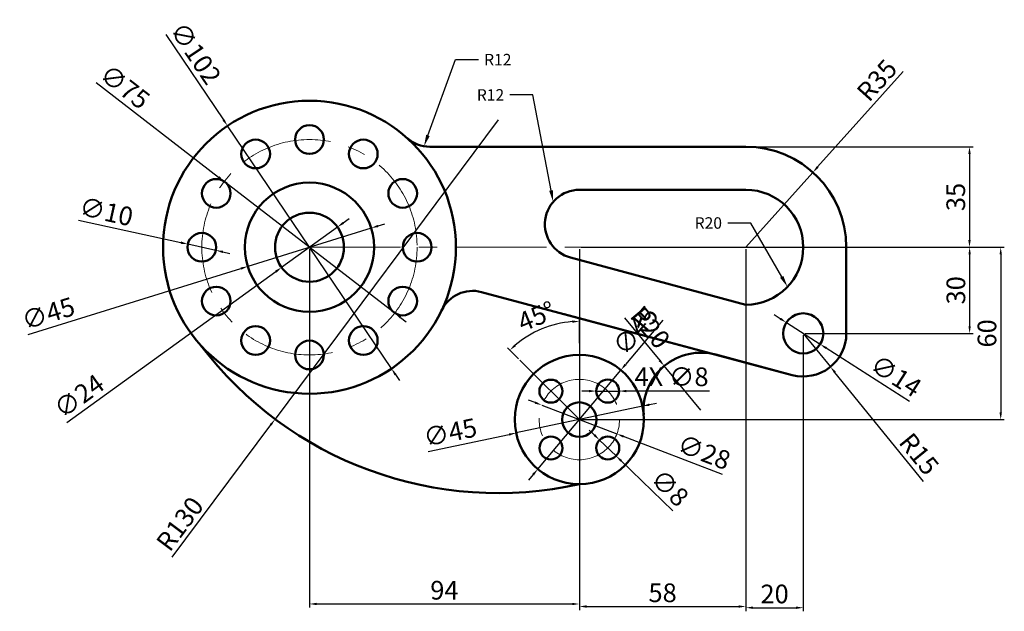
# Model space of a CAD drawing. Units: millimetres. Extents: x 3100 to 3443, y 1438 to 1644.
import ezdxf
from ezdxf import colors
from ezdxf.entities.mleader import LeaderData, LeaderLine
from ezdxf.math import Vec2, Vec3

# ---------------------------------------------------------------- set-up
doc = ezdxf.new("R2010")
doc.units = ezdxf.units.MM
doc.linetypes.add('CENTER', pattern=[50.8, 31.75, -6.35, 6.35, -6.35])
for name, color, linetype, lineweight in [('M-CNTR', 240, 'CENTER', 18), ('M-DIMS', 2, 'Continuous', 25), ('M-OUTL', 7, 'Continuous', 50)]:
    doc.layers.add(name, color=color, linetype=linetype, lineweight=lineweight)
doc.styles.get("Standard").update_dxf_attribs({"font": 'arial.ttf'})
doc.dimstyles.new('ISO-25', dxfattribs={"dimtxt": 6.5, "dimasz": 2.5, "dimexe": 1.25, "dimexo": 0.625, "dimtad": 1, "dimtxsty": 'Standard', "dimcen": 2.5, "dimadec": 0, "dimazin": 0, "dimtfac": 1, "dimtmove": 0, "dimatfit": 3, "dimfxl": 1, "dimarcsym": 0})

# ---------------------------------------------------------------- blocks, each defined once
blk = doc.blocks.new('*D1')
at = {"layer": 'Defpoints', "color": 0, "transparency": 16777216}
for p in [(3372.48, 1564.51), (3372.48, 1534.51), (3430.43, 1534.51)]:
    blk.add_point(p, dxfattribs=at)
at = {"layer": 'M-DIMS', "color": 0, "lineweight": -2, "transparency": 16777216}
for p, q in [((3373.1, 1564.51), (3431.68, 1564.51)), ((3430.43, 1562.01), (3430.43, 1537.01)), ((3373.1, 1534.51), (3431.68, 1534.51))]:
    blk.add_line(p, q, dxfattribs=at)
at = {"layer": 'M-DIMS', "color": 0, "transparency": 16777216}
for points in [[(3430.01, 1562.01), (3430.84, 1562.01), (3430.43, 1564.51)], [(3430.01, 1537.01), (3430.84, 1537.01), (3430.43, 1534.51)]]:
    blk.add_solid(points, dxfattribs=at)
at = {"layer": 'M-DIMS', "color": 0, "transparency": 16777216, "insert": (3426.48, 1549.51), "char_height": 6.5, "attachment_point": 5, "rotation": 90}
blk.add_mtext('30', dxfattribs=at)
blk = doc.blocks.new('*D2')
at = {"layer": 'Defpoints', "color": 0, "transparency": 16777216}
for p in [(3352.48, 1564.51), (3372.48, 1534.51), (3372.48, 1438.99)]:
    blk.add_point(p, dxfattribs=at)
at = {"layer": 'M-DIMS', "color": 0, "lineweight": -2, "transparency": 16777216}
for p, q in [((3352.48, 1563.88), (3352.48, 1437.74)), ((3372.48, 1533.88), (3372.48, 1437.74)), ((3354.98, 1438.99), (3369.98, 1438.99))]:
    blk.add_line(p, q, dxfattribs=at)
at = {"layer": 'M-DIMS', "color": 0, "transparency": 16777216}
for points in [[(3354.98, 1439.41), (3354.98, 1438.58), (3352.48, 1438.99)], [(3369.98, 1439.41), (3369.98, 1438.58), (3372.48, 1438.99)]]:
    blk.add_solid(points, dxfattribs=at)
at = {"layer": 'M-DIMS', "color": 0, "transparency": 16777216, "insert": (3362.48, 1442.94), "char_height": 6.5, "attachment_point": 5}
blk.add_mtext('20', dxfattribs=at)
blk = doc.blocks.new('*D3')
at = {"layer": 'Defpoints', "color": 0, "transparency": 16777216}
for p in [(3331.88, 1599.51), (3352.09, 1564.51), (3430.38, 1564.51)]:
    blk.add_point(p, dxfattribs=at)
at = {"layer": 'M-DIMS', "color": 0, "lineweight": -2, "transparency": 16777216}
for p, q in [((3332.51, 1599.51), (3431.63, 1599.51)), ((3430.38, 1597.01), (3430.38, 1567.01)), ((3352.72, 1564.51), (3431.63, 1564.51))]:
    blk.add_line(p, q, dxfattribs=at)
at = {"layer": 'M-DIMS', "color": 0, "transparency": 16777216}
for points in [[(3429.97, 1597.01), (3430.8, 1597.01), (3430.38, 1599.51)], [(3429.97, 1567.01), (3430.8, 1567.01), (3430.38, 1564.51)]]:
    blk.add_solid(points, dxfattribs=at)
at = {"layer": 'M-DIMS', "color": 0, "transparency": 16777216, "insert": (3426.44, 1582.01), "char_height": 6.5, "attachment_point": 5, "rotation": 90}
blk.add_mtext('35', dxfattribs=at)
blk = doc.blocks.new('*D4')
at = {"layer": 'Defpoints', "color": 0, "transparency": 16777216}
for p in [(3171.92, 1606.77), (3229.03, 1522.25)]:
    blk.add_point(p, dxfattribs=at)
at = {"layer": 'M-DIMS', "color": 0, "lineweight": -2, "transparency": 16777216}
for p, q in [((3150.4, 1638.62), (3170.53, 1608.84)), ((3229.03, 1522.25), (3171.92, 1606.77)), ((3230.43, 1520.18), (3231.83, 1518.11))]:
    blk.add_line(p, q, dxfattribs=at)
at = {"layer": 'M-DIMS', "color": 0, "transparency": 16777216}
for points in [[(3170.87, 1609.07), (3170.18, 1608.6), (3171.92, 1606.77)], [(3230.77, 1520.41), (3230.08, 1519.94), (3229.03, 1522.25)]]:
    blk.add_solid(points, dxfattribs=at)
at = {"layer": 'M-DIMS', "color": 0, "transparency": 16777216, "insert": (3160.15, 1631.56), "char_height": 6.5, "attachment_point": 5, "rotation": 304.0444}
blk.add_mtext('∅102', dxfattribs=at)
blk = doc.blocks.new('*D5')
at = {"layer": 'Defpoints', "color": 0, "transparency": 16777216}
for p in [(3170.78, 1587.41), (3230.17, 1541.61)]:
    blk.add_point(p, dxfattribs=at)
at = {"layer": 'M-DIMS', "color": 0, "lineweight": -2, "transparency": 16777216}
for p, q in [((3126.15, 1621.82), (3168.8, 1588.93)), ((3230.17, 1541.61), (3170.78, 1587.41)), ((3232.15, 1540.08), (3234.13, 1538.55))]:
    blk.add_line(p, q, dxfattribs=at)
at = {"layer": 'M-DIMS', "color": 0, "transparency": 16777216}
for points in [[(3169.06, 1589.26), (3168.55, 1588.6), (3170.78, 1587.41)], [(3232.41, 1540.41), (3231.9, 1539.75), (3230.17, 1541.61)]]:
    blk.add_solid(points, dxfattribs=at)
at = {"layer": 'M-DIMS', "color": 0, "transparency": 16777216, "insert": (3135.67, 1619.69), "char_height": 6.5, "attachment_point": 5, "rotation": 322.3623}
blk.add_mtext('∅75', dxfattribs=at)
blk = doc.blocks.new('*D6')
at = {"layer": 'Defpoints', "color": 0, "transparency": 16777216}
for p in [(3158.09, 1565.58), (3167.86, 1563.43)]:
    blk.add_point(p, dxfattribs=at)
at = {"layer": 'M-DIMS', "color": 0, "lineweight": -2, "transparency": 16777216}
for p, q in [((3120.04, 1573.96), (3155.65, 1566.12)), ((3167.86, 1563.43), (3158.09, 1565.58)), ((3170.3, 1562.9), (3172.74, 1562.36))]:
    blk.add_line(p, q, dxfattribs=at)
at = {"layer": 'M-DIMS', "color": 0, "transparency": 16777216}
for points in [[(3155.74, 1566.53), (3155.56, 1565.71), (3158.09, 1565.58)], [(3170.39, 1563.3), (3170.21, 1562.49), (3167.86, 1563.43)]]:
    blk.add_solid(points, dxfattribs=at)
at = {"layer": 'M-DIMS', "color": 0, "transparency": 16777216, "insert": (3129.53, 1576.1), "char_height": 6.5, "attachment_point": 5, "rotation": 347.5819}
blk.add_mtext('∅10', dxfattribs=at)
blk = doc.blocks.new('*D7')
at = {"layer": 'Defpoints', "color": 0, "transparency": 16777216}
for p in [(3221.96, 1571.18), (3178.99, 1557.84)]:
    blk.add_point(p, dxfattribs=at)
at = {"layer": 'M-DIMS', "color": 0, "lineweight": -2, "transparency": 16777216}
for p, q in [((3221.96, 1571.18), (3178.99, 1557.84)), ((3224.35, 1571.92), (3226.74, 1572.66)), ((3102.51, 1534.1), (3176.6, 1557.1))]:
    blk.add_line(p, q, dxfattribs=at)
at = {"layer": 'M-DIMS', "color": 0, "transparency": 16777216}
for points in [[(3224.23, 1572.32), (3224.48, 1571.52), (3221.96, 1571.18)], [(3176.48, 1557.49), (3176.72, 1556.7), (3178.99, 1557.84)]]:
    blk.add_solid(points, dxfattribs=at)
at = {"layer": 'M-DIMS', "color": 0, "transparency": 16777216, "insert": (3109.73, 1540.66), "char_height": 6.5, "attachment_point": 5, "rotation": 17.2442}
blk.add_mtext('∅45', dxfattribs=at)
blk = doc.blocks.new('*D8')
at = {"layer": 'Defpoints', "color": 0, "transparency": 16777216}
for p in [(3210.21, 1571.53), (3190.75, 1557.48)]:
    blk.add_point(p, dxfattribs=at)
at = {"layer": 'M-DIMS', "color": 0, "lineweight": -2, "transparency": 16777216}
for p, q in [((3212.23, 1572.99), (3214.26, 1574.46)), ((3210.21, 1571.53), (3190.75, 1557.48)), ((3115.96, 1503.5), (3188.72, 1556.02))]:
    blk.add_line(p, q, dxfattribs=at)
at = {"layer": 'M-DIMS', "color": 0, "transparency": 16777216}
for points in [[(3211.99, 1573.33), (3212.48, 1572.66), (3210.21, 1571.53)], [(3188.48, 1556.36), (3188.96, 1555.68), (3190.75, 1557.48)]]:
    blk.add_solid(points, dxfattribs=at)
at = {"layer": 'M-DIMS', "color": 0, "transparency": 16777216, "insert": (3120.68, 1512), "char_height": 6.5, "attachment_point": 5, "rotation": 35.823}
blk.add_mtext('∅24', dxfattribs=at)
blk = doc.blocks.new('*D9')
at = {"layer": 'Defpoints', "color": 0, "transparency": 16777216}
for p in [(3266.19, 1608.89), (3188.49, 1504.67)]:
    blk.add_point(p, dxfattribs=at)
at = {"layer": 'M-DIMS', "color": 0, "lineweight": -2, "transparency": 16777216}
for p, q in [((3266.19, 1608.89), (3188.49, 1504.67)), ((3152.65, 1456.59), (3186.99, 1502.66))]:
    blk.add_line(p, q, dxfattribs=at)
at = {"layer": 'M-DIMS', "color": 0, "transparency": 16777216}
blk.add_solid([(3186.66, 1502.91), (3187.33, 1502.41), (3188.49, 1504.67)], dxfattribs=at)
at = {"layer": 'M-DIMS', "color": 0, "transparency": 16777216, "insert": (3156, 1467.69), "char_height": 6.5, "attachment_point": 5, "rotation": 53.2956}
blk.add_mtext('R130', dxfattribs=at)
blk = doc.blocks.new('*D10')
at = {"layer": 'Defpoints', "color": 0, "transparency": 16777216}
for p in [(3375.82, 1590.58), (3352.48, 1564.51)]:
    blk.add_point(p, dxfattribs=at)
at = {"layer": 'M-DIMS', "color": 0, "lineweight": -2, "transparency": 16777216}
for p, q in [((3407.31, 1625.75), (3377.49, 1592.45)), ((3352.48, 1564.51), (3375.82, 1590.58))]:
    blk.add_line(p, q, dxfattribs=at)
at = {"layer": 'M-DIMS', "color": 0, "transparency": 16777216}
blk.add_solid([(3377.18, 1592.72), (3377.8, 1592.17), (3375.82, 1590.58)], dxfattribs=at)
at = {"layer": 'M-DIMS', "color": 0, "transparency": 16777216, "insert": (3398.76, 1622.11), "char_height": 6.5, "attachment_point": 5, "rotation": 48.1595}
blk.add_mtext('R35', dxfattribs=at)
blk = doc.blocks.new('*D11')
at = {"layer": 'Defpoints', "color": 0, "transparency": 16777216}
for p in [(3285.62, 1537.52), (3294.48, 1530.53), (3273.7, 1525.24), (3294.48, 1504.51), (3294.48, 1504.51)]:
    blk.add_point(p, dxfattribs=at)
at = {"layer": 'M-DIMS', "color": 0, "lineweight": -2, "transparency": 16777216}
for p, q in [((3294.48, 1531.16), (3294.48, 1539.94)), ((3273.26, 1525.68), (3269.4, 1529.53))]:
    blk.add_line(p, q, dxfattribs=at)
blk.add_arc((3294.48, 1504.51), 34.18, 94.192, 130.8751, dxfattribs=at)
at = {"layer": 'M-DIMS', "color": 0, "transparency": 16777216}
for points in [[(3291.96, 1539.01), (3291.99, 1538.18), (3294.48, 1538.69)], [(3272.39, 1530.05), (3271.83, 1530.66), (3270.28, 1528.65)]]:
    blk.add_solid(points, dxfattribs=at)
at = {"layer": 'M-DIMS', "color": 0, "transparency": 16777216, "insert": (3279.87, 1539.71), "char_height": 6.5, "attachment_point": 5, "rotation": 22.5336}
blk.add_mtext('45°', dxfattribs=at)
blk = doc.blocks.new('*D12')
at = {"layer": 'Defpoints', "color": 0, "transparency": 16777216}
for p in [(3200.48, 1564.51), (3294.48, 1564.51), (3294.48, 1440.29)]:
    blk.add_point(p, dxfattribs=at)
at = {"layer": 'M-DIMS', "color": 0, "lineweight": -2, "transparency": 16777216}
for p, q in [((3200.48, 1563.88), (3200.48, 1439.04)), ((3294.48, 1563.88), (3294.48, 1439.04)), ((3202.98, 1440.29), (3291.98, 1440.29))]:
    blk.add_line(p, q, dxfattribs=at)
at = {"layer": 'M-DIMS', "color": 0, "transparency": 16777216}
for points in [[(3202.98, 1440.71), (3202.98, 1439.88), (3200.48, 1440.29)], [(3291.98, 1440.71), (3291.98, 1439.88), (3294.48, 1440.29)]]:
    blk.add_solid(points, dxfattribs=at)
at = {"layer": 'M-DIMS', "color": 0, "transparency": 16777216, "insert": (3247.48, 1444.24), "char_height": 6.5, "attachment_point": 5}
blk.add_mtext('94', dxfattribs=at)
blk = doc.blocks.new('*D13')
at = {"layer": 'Defpoints', "color": 0, "transparency": 16777216}
for p in [(3294.48, 1564.51), (3352.48, 1564.51), (3352.48, 1439.41)]:
    blk.add_point(p, dxfattribs=at)
at = {"layer": 'M-DIMS', "color": 0, "lineweight": -2, "transparency": 16777216}
for p, q in [((3294.48, 1563.88), (3294.48, 1438.16)), ((3352.48, 1563.88), (3352.48, 1438.16)), ((3296.98, 1439.41), (3349.98, 1439.41))]:
    blk.add_line(p, q, dxfattribs=at)
at = {"layer": 'M-DIMS', "color": 0, "transparency": 16777216}
for points in [[(3296.98, 1439.83), (3296.98, 1438.99), (3294.48, 1439.41)], [(3349.98, 1439.83), (3349.98, 1438.99), (3352.48, 1439.41)]]:
    blk.add_solid(points, dxfattribs=at)
at = {"layer": 'M-DIMS', "color": 0, "transparency": 16777216, "insert": (3323.48, 1443.35), "char_height": 6.5, "attachment_point": 5}
blk.add_mtext('58', dxfattribs=at)
blk = doc.blocks.new('*D14')
at = {"layer": 'Defpoints', "color": 0, "transparency": 16777216}
for p in [(3316.49, 1509.18), (3272.47, 1499.83)]:
    blk.add_point(p, dxfattribs=at)
at = {"layer": 'M-DIMS', "color": 0, "lineweight": -2, "transparency": 16777216}
for p, q in [((3316.49, 1509.18), (3272.47, 1499.83)), ((3318.93, 1509.7), (3321.38, 1510.22)), ((3241.87, 1493.33), (3270.02, 1499.31))]:
    blk.add_line(p, q, dxfattribs=at)
at = {"layer": 'M-DIMS', "color": 0, "transparency": 16777216}
for points in [[(3318.84, 1510.11), (3319.02, 1509.3), (3316.49, 1509.18)], [(3269.94, 1499.72), (3270.11, 1498.91), (3272.47, 1499.83)]]:
    blk.add_solid(points, dxfattribs=at)
at = {"layer": 'M-DIMS', "color": 0, "transparency": 16777216, "insert": (3249.66, 1499.2), "char_height": 6.5, "attachment_point": 5, "rotation": 11.9941}
blk.add_mtext('∅45', dxfattribs=at)
blk = doc.blocks.new('*D15')
at = {"layer": 'Defpoints', "color": 0, "transparency": 16777216}
for p in [(3301.5, 1497.39), (3307.27, 1491.85)]:
    blk.add_point(p, dxfattribs=at)
at = {"layer": 'M-DIMS', "color": 0, "lineweight": -2, "transparency": 16777216}
for p, q in [((3299.7, 1499.13), (3297.9, 1500.86)), ((3301.5, 1497.39), (3307.27, 1491.85)), ((3327.09, 1472.78), (3309.07, 1490.11))]:
    blk.add_line(p, q, dxfattribs=at)
at = {"layer": 'M-DIMS', "color": 0, "transparency": 16777216}
for points in [[(3299.99, 1499.43), (3299.41, 1498.83), (3301.5, 1497.39)], [(3309.36, 1490.41), (3308.78, 1489.81), (3307.27, 1491.85)]]:
    blk.add_solid(points, dxfattribs=at)
at = {"layer": 'M-DIMS', "color": 0, "transparency": 16777216, "insert": (3325.41, 1480.11), "char_height": 6.5, "attachment_point": 5, "rotation": 316.1062}
blk.add_mtext('∅8', dxfattribs=at)
blk = doc.blocks.new('*D16')
at = {"layer": 'Defpoints', "color": 0, "transparency": 16777216}
for p in [(3281.4, 1509.52), (3307.55, 1499.5)]:
    blk.add_point(p, dxfattribs=at)
at = {"layer": 'M-DIMS', "color": 0, "lineweight": -2, "transparency": 16777216}
for p, q in [((3279.07, 1510.42), (3276.74, 1511.31)), ((3281.4, 1509.52), (3307.55, 1499.5)), ((3344.38, 1485.37), (3309.88, 1498.6))]:
    blk.add_line(p, q, dxfattribs=at)
at = {"layer": 'M-DIMS', "color": 0, "transparency": 16777216}
for points in [[(3279.22, 1510.8), (3278.92, 1510.03), (3281.4, 1509.52)], [(3310.03, 1498.99), (3309.73, 1498.21), (3307.55, 1499.5)]]:
    blk.add_solid(points, dxfattribs=at)
at = {"layer": 'M-DIMS', "color": 0, "transparency": 16777216, "insert": (3337.62, 1492.38), "char_height": 6.5, "attachment_point": 5, "rotation": 339.0204}
blk.add_mtext('∅28', dxfattribs=at)
blk = doc.blocks.new('*D17')
at = {"layer": 'Defpoints', "color": 0, "transparency": 16777216}
for p in [(3294.48, 1564.51), (3294.48, 1504.51), (3441.26, 1504.51)]:
    blk.add_point(p, dxfattribs=at)
at = {"layer": 'M-DIMS', "color": 0, "lineweight": -2, "transparency": 16777216}
for p, q in [((3295.1, 1564.51), (3442.51, 1564.51)), ((3441.26, 1562.01), (3441.26, 1507.01)), ((3295.1, 1504.51), (3442.51, 1504.51))]:
    blk.add_line(p, q, dxfattribs=at)
at = {"layer": 'M-DIMS', "color": 0, "transparency": 16777216}
for points in [[(3440.84, 1562.01), (3441.67, 1562.01), (3441.26, 1564.51)], [(3440.84, 1507.01), (3441.67, 1507.01), (3441.26, 1504.51)]]:
    blk.add_solid(points, dxfattribs=at)
at = {"layer": 'M-DIMS', "color": 0, "transparency": 16777216, "insert": (3437.31, 1534.51), "char_height": 6.5, "attachment_point": 5, "rotation": 90}
blk.add_mtext('60', dxfattribs=at)
blk = doc.blocks.new('*D18')
at = {"layer": 'Defpoints', "color": 0, "transparency": 16777216}
for p in [(3372.48, 1534.51), (3381.94, 1522.87)]:
    blk.add_point(p, dxfattribs=at)
at = {"layer": 'M-DIMS', "color": 0, "lineweight": -2, "transparency": 16777216}
for p, q in [((3372.48, 1534.51), (3381.94, 1522.87)), ((3414.41, 1482.97), (3383.52, 1520.93))]:
    blk.add_line(p, q, dxfattribs=at)
at = {"layer": 'M-DIMS', "color": 0, "transparency": 16777216}
blk.add_solid([(3383.84, 1521.2), (3383.2, 1520.67), (3381.94, 1522.87)], dxfattribs=at)
at = {"layer": 'M-DIMS', "color": 0, "transparency": 16777216, "insert": (3412.16, 1491.99), "char_height": 6.5, "attachment_point": 5, "rotation": 309.136}
blk.add_mtext('R15', dxfattribs=at)
blk = doc.blocks.new('*D19')
at = {"layer": 'Defpoints', "color": 0, "transparency": 16777216}
for p in [(3366.58, 1538.28), (3378.37, 1530.73)]:
    blk.add_point(p, dxfattribs=at)
at = {"layer": 'M-DIMS', "color": 0, "lineweight": -2, "transparency": 16777216}
for p, q in [((3364.48, 1539.63), (3362.37, 1540.98)), ((3366.58, 1538.28), (3378.37, 1530.73)), ((3409.5, 1510.79), (3380.48, 1529.38))]:
    blk.add_line(p, q, dxfattribs=at)
at = {"layer": 'M-DIMS', "color": 0, "transparency": 16777216}
for points in [[(3364.7, 1539.98), (3364.25, 1539.28), (3366.58, 1538.28)], [(3380.7, 1529.73), (3380.25, 1529.03), (3378.37, 1530.73)]]:
    blk.add_solid(points, dxfattribs=at)
at = {"layer": 'M-DIMS', "color": 0, "transparency": 16777216, "insert": (3404.32, 1519.01), "char_height": 6.5, "attachment_point": 5, "rotation": 327.3601}
blk.add_mtext('∅14', dxfattribs=at)
blk = doc.blocks.new('INDEX-HOLE-D8')
blk.add_circle((4, 4), 4)
blk = doc.blocks.new('INDEX-HOLE-D10')
blk.add_circle((5, 5), 5)
blk = doc.blocks.new('*D22')
at = {"layer": 'Defpoints', "color": 0, "transparency": 16777216}
for p in [(3308.94, 1521.74), (3280.01, 1487.27)]:
    blk.add_point(p, dxfattribs=at)
at = {"layer": 'M-DIMS', "color": 0, "lineweight": -2, "transparency": 16777216}
for p, q in [((3323.52, 1539.12), (3310.55, 1523.66)), ((3280.01, 1487.27), (3308.94, 1521.74)), ((3278.41, 1485.36), (3276.8, 1483.44))]:
    blk.add_line(p, q, dxfattribs=at)
at = {"layer": 'M-DIMS', "color": 0, "transparency": 16777216}
for points in [[(3310.23, 1523.93), (3310.87, 1523.39), (3308.94, 1521.74)], [(3278.09, 1485.63), (3278.73, 1485.09), (3280.01, 1487.27)]]:
    blk.add_solid(points, dxfattribs=at)
at = {"layer": 'M-DIMS', "color": 0, "transparency": 16777216, "insert": (3314.68, 1535), "char_height": 6.5, "attachment_point": 5, "rotation": 49.9981}
blk.add_mtext('∅45', dxfattribs=at)
blk = doc.blocks.new('*D23')
at = {"layer": 'Defpoints', "color": 0, "transparency": 16777216}
for p in [(3300.36, 1514.42), (3308.36, 1514.42)]:
    blk.add_point(p, dxfattribs=at)
at = {"layer": 'M-DIMS', "color": 0, "lineweight": -2, "transparency": 16777216}
for p, q in [((3297.86, 1514.42), (3295.36, 1514.42)), ((3300.36, 1514.42), (3308.36, 1514.42)), ((3339.84, 1514.43), (3310.86, 1514.42))]:
    blk.add_line(p, q, dxfattribs=at)
at = {"layer": 'M-DIMS', "color": 0, "transparency": 16777216}
for points in [[(3297.86, 1514.83), (3297.86, 1514), (3300.36, 1514.42)], [(3310.86, 1514.84), (3310.86, 1514), (3308.36, 1514.42)]]:
    blk.add_solid(points, dxfattribs=at)
at = {"layer": 'M-DIMS', "color": 0, "transparency": 16777216, "insert": (3326.6, 1518.55), "char_height": 6.5, "attachment_point": 5, "rotation": 0.0139}
blk.add_mtext('4X ∅8', dxfattribs=at)
blk = doc.blocks.new('*D24')
at = {"layer": 'Defpoints', "color": 0, "transparency": 16777216}
for p in [(3324.06, 1523.17), (3336.85, 1507.79)]:
    blk.add_point(p, dxfattribs=at)
at = {"layer": 'M-DIMS', "color": 0, "lineweight": -2, "transparency": 16777216}
for p, q in [((3310.15, 1539.9), (3322.46, 1525.1)), ((3336.85, 1507.79), (3324.06, 1523.17))]:
    blk.add_line(p, q, dxfattribs=at)
at = {"layer": 'M-DIMS', "color": 0, "transparency": 16777216}
blk.add_solid([(3322.78, 1525.36), (3322.14, 1524.83), (3324.06, 1523.17)], dxfattribs=at)
at = {"layer": 'M-DIMS', "color": 0, "transparency": 16777216, "insert": (3318.54, 1535.98), "char_height": 6.5, "attachment_point": 5, "rotation": 309.7425}
blk.add_mtext('R20', dxfattribs=at)

msp = doc.modelspace()

# ---------------------------------------------------------------- linework, layer by layer
at = {"layer": 'M-CNTR'}
for p, q in [((3200.476, 1564.508), (3294.476, 1564.508)), ((3294.476, 1564.508), (3352.476, 1564.508)), ((3352.476, 1564.508), (3372.476, 1564.508)), ((3372.476, 1564.508), (3393.392, 1564.508)), ((3294.476, 1504.508), (3294.476, 1530.533)), ((3294.476, 1504.508), (3273.698, 1525.238))]:
    msp.add_line(p, q, dxfattribs=at)
for centre, radius in [((3200.476, 1564.508), 37.5), ((3294.476, 1504.508), 14)]:
    msp.add_circle(centre, radius, dxfattribs=at)
at = {"layer": 'M-OUTL'}
for p, q in [((3352.476, 1599.508), (3242.429, 1599.508)), ((3294.476, 1599.508), (3352.476, 1599.508)), ((3294.476, 1584.508), (3352.476, 1584.508)), ((3387.476, 1564.508), (3387.476, 1534.508)), ((3291.364, 1560.919), (3352.476, 1544.508)), ((3260.4, 1548.906), (3368.607, 1520.016)), ((3289.158, 1541.228), (3368.607, 1520.016)), ((3368.607, 1520.016), (3342.008, 1527.117))]:
    msp.add_line(p, q, dxfattribs=at)
for centre, radius in [((3200.476, 1564.508), 51), ((3200.476, 1564.508), 22.5), ((3200.476, 1564.508), 12), ((3372.476, 1534.508), 7), ((3294.476, 1504.508), 22.5), ((3294.476, 1504.508), 6)]:
    msp.add_circle(centre, radius, dxfattribs=at)
for centre, radius, start, end in [((3242.429, 1611.508), 12, 228.24779, 270), ((3352.476, 1564.508), 35, 0, 90), ((3294.476, 1572.508), 12, 90, 254.96883), ((3352.476, 1564.508), 20, 270, 90), ((3257.304, 1537.312), 12, 75.05106, 154.42613), ((3372.476, 1534.508), 15, 255.05106, 0), ((3266.187, 1608.893), 130, 217.13589, 282.56863), ((3336.849, 1507.794), 20, 75.05106, 184.43473)]:
    msp.add_arc(centre, radius, start, end, dxfattribs=at)

# ---------------------------------------------------------------- block references
for name, p in [('INDEX-HOLE-D10', (3195.476, 1597.008)), ('INDEX-HOLE-D10', (3176.726, 1591.984)), ('INDEX-HOLE-D10', (3214.226, 1591.984)), ('INDEX-HOLE-D10', (3163, 1578.258)), ('INDEX-HOLE-D10', (3227.952, 1578.258)), ('INDEX-HOLE-D10', (3157.976, 1559.508)), ('INDEX-HOLE-D10', (3232.976, 1559.508)), ('INDEX-HOLE-D10', (3163, 1540.758)), ('INDEX-HOLE-D10', (3227.952, 1540.758)), ('INDEX-HOLE-D10', (3176.726, 1527.032)), ('INDEX-HOLE-D10', (3214.226, 1527.032)), ('INDEX-HOLE-D10', (3195.476, 1522.008)), ('INDEX-HOLE-D8', (3280.565, 1510.396)), ('INDEX-HOLE-D8', (3300.364, 1510.419)), ('INDEX-HOLE-D8', (3280.588, 1490.597)), ('INDEX-HOLE-D8', (3300.387, 1490.62))]:
    msp.add_blockref(name, p, dxfattribs=at)

# ---------------------------------------------------------------- dimensions: what is measured, and where the dimension line sits
at = {"layer": 'M-DIMS'}
for p1, p2, override, picture, middle in [((3229.028, 1522.249), (3171.925, 1606.767), {"dimclrd": 0, "dimclre": 0, "dimclrt": 0}, '*D4', (3156.735, 1629.248)), ((3230.172, 1541.608), (3170.78, 1587.408), {"dimclrd": 0, "dimclre": 0, "dimclrt": 0}, '*D5', (3133.151, 1616.426)), ((3167.859, 1563.433), (3158.093, 1565.583), {"dimclrd": 0, "dimclre": 0, "dimclrt": 0}, '*D6', (3128.642, 1572.068)), ((3210.206, 1571.531), (3190.746, 1557.485), {"dimclrd": 0, "dimclre": 0, "dimclrt": 0}, '*D8', (3123.093, 1508.65)), ((3221.965, 1571.178), (3178.988, 1557.838), {"dimclrd": 0, "dimclre": 0, "dimclrt": 0}, '*D7', (3110.954, 1536.72)), ((3280.013, 1487.272), (3308.94, 1521.743), {"dimdec": 0, "dimlfac": 1, "dimrnd": 0, "dimzin": 0, "dimdsep": 46, "dimlunit": 2}, '*D22', (3317.837, 1532.346)), ((3366.582, 1538.283), (3378.371, 1530.732), {"dimclrd": 0, "dimclre": 0, "dimclrt": 0}, '*D19', (3402.092, 1515.539)), ((3316.485, 1509.184), (3272.467, 1499.832), {"dimclrd": 0, "dimclre": 0, "dimclrt": 0}, '*D14', (3250.519, 1495.169)), ((3281.404, 1509.52), (3307.548, 1499.495), {"dimclrd": 0, "dimclre": 0, "dimclrt": 0}, '*D16', (3336.143, 1488.53)), ((3301.505, 1497.393), (3307.27, 1491.847), {"dimclrd": 0, "dimclre": 0, "dimclrt": 0}, '*D15', (3322.554, 1477.142))]:
    dim = msp.add_diameter_dim_2p(p1=p1, p2=p2, dimstyle='ISO-25', override=override, dxfattribs=at)
    dim.commit()
    dim.dimension.update_dxf_attribs({"geometry": picture, "text_midpoint": middle, "dimtype": 163})
for center, mpoint, picture, middle in [((3352.476, 1564.508), (3375.823, 1590.583), '*D10', (3401.697, 1619.48)), ((3266.187, 1608.893), (3188.488, 1504.668), '*D9', (3159.163, 1465.332)), ((3372.476, 1534.508), (3381.944, 1522.873), '*D18', (3409.101, 1489.499))]:
    dim = msp.add_radius_dim(center=center, mpoint=mpoint, dimstyle='ISO-25', override={"dimclrd": 0, "dimclre": 0, "dimclrt": 0}, dxfattribs=at)
    dim.commit()
    dim.dimension.update_dxf_attribs({"geometry": picture, "text_midpoint": middle, "dimtype": 164})
for base, p1, p2, picture, middle in [((3430.382, 1564.508), (3331.883, 1599.508), (3352.091, 1564.508), '*D3', (3426.436, 1582.008)), ((3441.257, 1504.508), (3294.476, 1564.508), (3294.476, 1504.508), '*D17', (3437.313, 1534.508)), ((3430.425, 1534.508), (3372.476, 1564.508), (3372.476, 1534.508), '*D1', (3426.48, 1549.508))]:
    dim = msp.add_linear_dim(base=base, p1=p1, p2=p2, angle=90, dimstyle='ISO-25', override={"dimclrd": 0, "dimclre": 0, "dimclrt": 0}, dxfattribs=at)
    dim.commit()
    dim.dimension.update_dxf_attribs({"geometry": picture, "text_midpoint": middle})
for base, p1, p2, picture, middle in [((3294.476, 1440.293), (3200.476, 1564.508), (3294.476, 1564.508), '*D12', (3247.476, 1444.237)), ((3352.476, 1439.411), (3294.476, 1564.508), (3352.476, 1564.508), '*D13', (3323.476, 1443.355)), ((3372.476, 1438.994), (3352.476, 1564.508), (3372.476, 1534.508), '*D2', (3362.476, 1442.938))]:
    dim = msp.add_linear_dim(base=base, p1=p1, p2=p2, dimstyle='ISO-25', override={"dimclrd": 0, "dimclre": 0, "dimclrt": 0}, dxfattribs=at)
    dim.commit()
    dim.dimension.update_dxf_attribs({"geometry": picture, "text_midpoint": middle})
dim = msp.add_angular_dim_2l(base=(3285.618, 1537.517), line1=((3294.476, 1504.508), (3294.476, 1530.533)), line2=((3294.476, 1504.508), (3273.698, 1525.238)), dimstyle='ISO-25', override={"dimclrd": 0, "dimclre": 0, "dimclrt": 0}, dxfattribs=at)
dim.commit()
dim.dimension.update_dxf_attribs({"geometry": '*D11', "text_midpoint": (3279.872, 1539.707)})
dim = msp.add_radius_dim(center=(3336.849, 1507.794), mpoint=(3324.062, 1523.173), dimstyle='ISO-25', override={"dimdec": 0, "dimlfac": 1, "dimrnd": 0, "dimzin": 0, "dimdsep": 46, "dimlunit": 2}, dxfattribs=at)
dim.commit()
dim.dimension.update_dxf_attribs({"geometry": '*D24', "text_midpoint": (3318.54, 1535.982)})
dim = msp.add_diameter_dim_2p(p1=(3300.364, 1514.418), p2=(3308.364, 1514.42), text='4X <>', dimstyle='ISO-25', override={"dimdec": 0, "dimlfac": 1, "dimrnd": 0, "dimzin": 0, "dimdsep": 46, "dimlunit": 2}, dxfattribs=at)
dim.commit()
dim.dimension.update_dxf_attribs({"geometry": '*D23', "text_midpoint": (3326.603, 1514.424), "dimtype": 163})

# ---------------------------------------------------------------- leaders
ml = msp.add_multileader_mtext('Standard', dxfattribs=at)
ml.set_content('R12', color=256)
ml.set_leader_properties()
ml.build(insert=Vec2(0, 0))
ctx = ml.context
ctx.base_point, ctx.plane_origin = Vec3(3259.31, 1629.831), Vec3(3240.377, 1599.685)
notes = []
notes.append((ctx, [(0, (1, 1, 0), (3251.31, 1629.831), (1, 0), 8, [(0, [(3240.377, 1599.685)], 0, [])])]))
ctx.mtext.insert, ctx.mtext.flow_direction = Vec3(3261.31, 1631.831), 5
ml = msp.add_multileader_mtext('Standard', dxfattribs=at)
ml.set_content('R12', color=256)
ml.set_leader_properties()
ml.build(insert=Vec2(0, 0))
ctx = ml.context
ctx.base_point, ctx.plane_origin = Vec3(3256.777, 1617.545), Vec3(3285.37, 1580.323)
ctx.text_align_type = 2
notes.append((ctx, [(0, (1, 1, 0), (3278.294, 1617.545), (-1, 0), 8, [(0, [(3285.37, 1580.323)], 0, [])])]))
ctx.mtext.insert, ctx.mtext.alignment, ctx.mtext.flow_direction = Vec3(3268.294, 1619.545), 3, 5
ml = msp.add_multileader_mtext('Standard', dxfattribs=at)
ml.set_content('R20', color=256)
ml.set_leader_properties()
ml.build(insert=Vec2(0, 0))
ctx = ml.context
ctx.base_point, ctx.plane_origin = Vec3(3332.627, 1572.917), Vec3(3366.979, 1550.735)
ctx.text_align_type = 2
notes.append((ctx, [(0, (1, 1, 0), (3354.172, 1572.917), (-1, 0), 8, [(0, [(3366.979, 1550.735)], 0, [])])]))
ctx.mtext.insert, ctx.mtext.alignment, ctx.mtext.flow_direction = Vec3(3344.172, 1574.951), 3, 5
for ctx, leaders in notes:
    for number, flags, end, landing, length, lines in leaders:
        leader = LeaderData()
        leader.index, (leader.has_last_leader_line, leader.has_dogleg_vector, leader.attachment_direction) = number, flags
        leader.last_leader_point, leader.dogleg_vector, leader.dogleg_length = Vec3(end), Vec3(landing), length
        for number, points, colour, breaks in lines:
            line = LeaderLine()
            line.index, line.vertices, line.color, line.breaks = number, Vec3.list(points), colors.encode_raw_color(colour), breaks
            leader.lines.append(line)
        ctx.leaders.append(leader)

doc.saveas('drawing.dxf')
